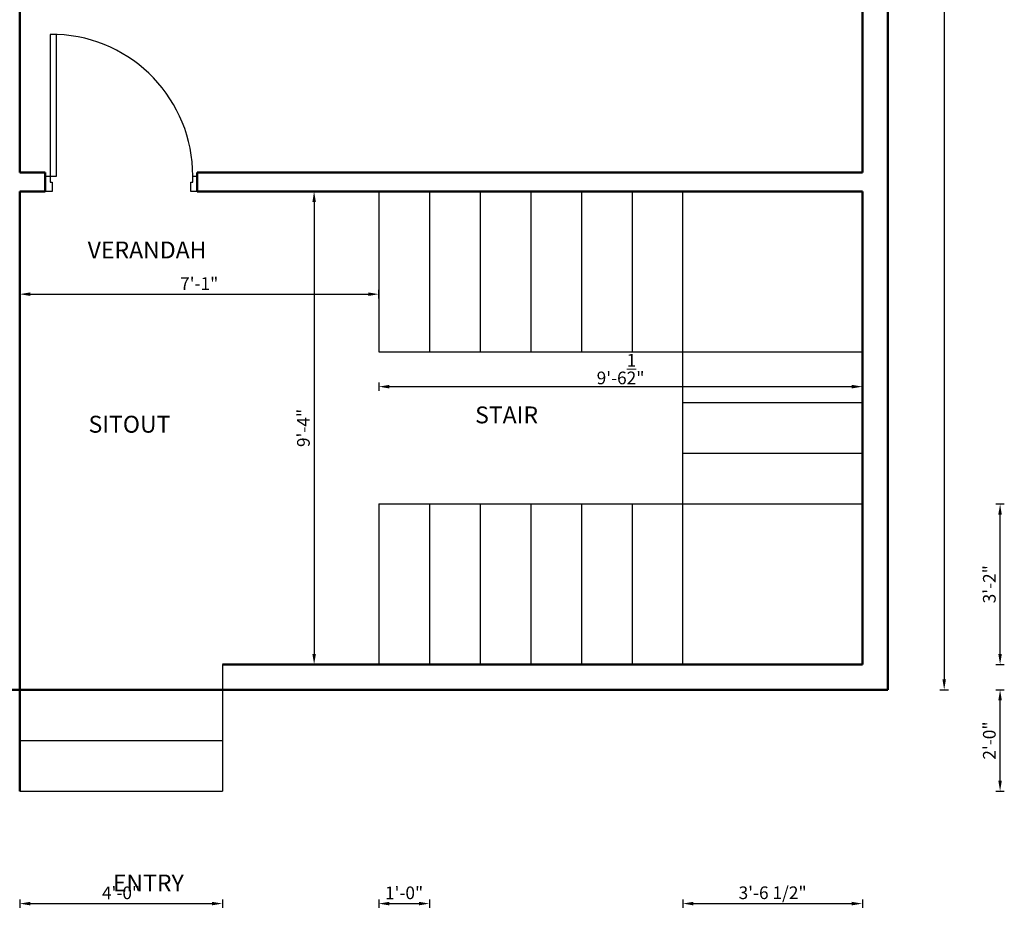
# Model space of a CAD drawing. Units: inches. Extents: x 1961 to 3038, y 800 to 1438.
# Tile 6 of 13: x 2803 to 3036, y 800 to 1012. Entities that reach past the tile are written whole.
import ezdxf

# ---------------------------------------------------------------- set-up
doc = ezdxf.new("R2010")
doc.units = ezdxf.units.IN
for name, color, linetype, lineweight in [('A-ANNO-DIMS', 2, 'Continuous', 18), ('A-ANNO-TEXT', 7, 'Continuous', 25), ('A-AREA-IDEN', 7, 'Continuous', 25), ('A-DOOR', 3, 'Continuous', 25), ('A-FLOR-STRS', 7, 'Continuous', 25), ('A-WALL', 7, 'Continuous', 50)]:
    doc.layers.add(name, color=color, linetype=linetype, lineweight=lineweight)
doc.styles.get("Standard").update_dxf_attribs({"font": 'arial.ttf'})
doc.dimstyles.new('ISO-25', dxfattribs={"dimtxt": 3, "dimasz": 2.5, "dimexe": 1, "dimexo": 1, "dimtad": 1, "dimdec": 4, "dimlunit": 4, "dimtxsty": 'Standard', "dimcen": 2.5, "dimadec": 0, "dimazin": 0, "dimtfac": 1, "dimtdec": 4, "dimtmove": 0, "dimatfit": 3, "dimfxl": 1, "dimfxlon": 1, "dimarcsym": 0})

# ---------------------------------------------------------------- blocks, each defined once
blk = doc.blocks.new('*D6')
at = {"layer": 'A-ANNO-DIMS', "color": 0, "lineweight": -2, "transparency": 16777216}
for p, q in [((2873.97, 970.92), (2871.97, 970.92)), ((2872.97, 968.42), (2872.97, 861.42)), ((2873.97, 858.92), (2871.97, 858.92))]:
    blk.add_line(p, q, dxfattribs=at)
at = {"layer": 'A-ANNO-DIMS', "color": 0, "transparency": 16777216}
for points in [[(2872.56, 968.42), (2873.39, 968.42), (2872.97, 970.92)], [(2872.56, 861.42), (2873.39, 861.42), (2872.97, 858.92)]]:
    blk.add_solid(points, dxfattribs=at)
at = {"layer": 'Defpoints', "color": 0, "transparency": 16777216}
for p in [(2888.27, 970.92), (2872.97, 858.92), (2888.27, 858.92)]:
    blk.add_point(p, dxfattribs=at)
at = {"layer": 'A-ANNO-DIMS', "color": 0, "transparency": 16777216, "insert": (2870.82, 914.92), "char_height": 3, "attachment_point": 5, "rotation": 90}
blk.add_mtext('9\'-4"', dxfattribs=at)
blk = doc.blocks.new('*D7')
at = {"layer": 'A-ANNO-DIMS', "color": 0, "lineweight": -2, "transparency": 16777216}
for p, q in [((2803.27, 945.9), (2803.27, 947.59)), ((2805.77, 946.59), (2885.77, 946.59)), ((2888.27, 945.59), (2888.27, 947.59))]:
    blk.add_line(p, q, dxfattribs=at)
at = {"layer": 'A-ANNO-DIMS', "color": 0, "transparency": 16777216}
for points in [[(2805.77, 947.01), (2805.77, 946.17), (2803.27, 946.59)], [(2885.77, 947.01), (2885.77, 946.17), (2888.27, 946.59)]]:
    blk.add_solid(points, dxfattribs=at)
at = {"layer": 'Defpoints', "color": 0, "transparency": 16777216}
for p in [(2888.27, 946.59), (2803.27, 944.9), (2888.27, 943.36)]:
    blk.add_point(p, dxfattribs=at)
at = {"layer": 'A-ANNO-DIMS', "color": 0, "transparency": 16777216, "insert": (2845.77, 948.72), "char_height": 3, "attachment_point": 5}
blk.add_mtext('7\'-1"', dxfattribs=at)
blk = doc.blocks.new('*D8')
at = {"layer": 'A-ANNO-DIMS', "color": 0, "lineweight": -2, "transparency": 16777216}
for p, q in [((2888.27, 925.7), (2888.27, 923.7)), ((3002.77, 925.7), (3002.77, 923.7)), ((2890.77, 924.7), (3000.27, 924.7))]:
    blk.add_line(p, q, dxfattribs=at)
at = {"layer": 'A-ANNO-DIMS', "color": 0, "transparency": 16777216}
for points in [[(2890.77, 925.12), (2890.77, 924.28), (2888.27, 924.7)], [(3000.27, 925.12), (3000.27, 924.28), (3002.77, 924.7)]]:
    blk.add_solid(points, dxfattribs=at)
at = {"layer": 'Defpoints', "color": 0, "transparency": 16777216}
for p in [(2888.27, 932.92), (3002.77, 932.92), (3002.77, 924.7)]:
    blk.add_point(p, dxfattribs=at)
at = {"layer": 'A-ANNO-DIMS', "color": 0, "transparency": 16777216, "insert": (2945.52, 928.86), "char_height": 3, "attachment_point": 5}
blk.add_mtext('9\'-6{\\H1x;\\S1/2;}"', dxfattribs=at)
blk = doc.blocks.new('*D26')
at = {"layer": 'A-ANNO-DIMS', "color": 0, "lineweight": -2, "transparency": 16777216}
for p, q in [((3021.14, 1314.92), (3023.14, 1314.92)), ((3022.14, 1312.42), (3022.14, 855.42)), ((3021.14, 852.92), (3023.14, 852.92))]:
    blk.add_line(p, q, dxfattribs=at)
at = {"layer": 'A-ANNO-DIMS', "color": 0, "transparency": 16777216}
for points in [[(3021.72, 1312.42), (3022.55, 1312.42), (3022.14, 1314.92)], [(3021.72, 855.42), (3022.55, 855.42), (3022.14, 852.92)]]:
    blk.add_solid(points, dxfattribs=at)
at = {"layer": 'Defpoints', "color": 0, "transparency": 16777216}
for p in [(3008.77, 1314.92), (3008.77, 852.92), (3022.14, 852.92)]:
    blk.add_point(p, dxfattribs=at)
at = {"layer": 'A-ANNO-DIMS', "color": 0, "transparency": 16777216, "insert": (3019.98, 1083.92), "char_height": 3, "attachment_point": 5, "rotation": 90}
blk.add_mtext('38\'-6"', dxfattribs=at)
blk = doc.blocks.new('*D71')
at = {"layer": 'A-ANNO-DIMS', "color": 0, "lineweight": -2, "transparency": 16777216}
for p, q in [((2803.27, 803.32), (2803.27, 801.32)), ((2805.77, 802.32), (2848.77, 802.32)), ((2851.27, 803.32), (2851.27, 801.32))]:
    blk.add_line(p, q, dxfattribs=at)
at = {"layer": 'A-ANNO-DIMS', "color": 0, "transparency": 16777216}
for points in [[(2805.77, 802.74), (2805.77, 801.9), (2803.27, 802.32)], [(2848.77, 802.74), (2848.77, 801.9), (2851.27, 802.32)]]:
    blk.add_solid(points, dxfattribs=at)
at = {"layer": 'Defpoints', "color": 0, "transparency": 16777216}
for p in [(2803.27, 828.92), (2851.27, 828.92), (2851.27, 802.32)]:
    blk.add_point(p, dxfattribs=at)
at = {"layer": 'A-ANNO-DIMS', "color": 0, "transparency": 16777216, "insert": (2827.27, 804.48), "char_height": 3, "attachment_point": 5}
blk.add_mtext('4\'-0"', dxfattribs=at)
blk = doc.blocks.new('*D72')
at = {"layer": 'A-ANNO-DIMS', "color": 0, "lineweight": -2, "transparency": 16777216}
for p, q in [((3034.37, 852.92), (3036.37, 852.92)), ((3035.37, 831.42), (3035.37, 850.42)), ((3034.37, 828.92), (3036.37, 828.92))]:
    blk.add_line(p, q, dxfattribs=at)
at = {"layer": 'A-ANNO-DIMS', "color": 0, "transparency": 16777216}
for points in [[(3034.95, 850.42), (3035.78, 850.42), (3035.37, 852.92)], [(3034.95, 831.42), (3035.78, 831.42), (3035.37, 828.92)]]:
    blk.add_solid(points, dxfattribs=at)
at = {"layer": 'Defpoints', "color": 0, "transparency": 16777216}
for p in [(3008.77, 852.92), (3035.37, 852.92), (2851.27, 828.92)]:
    blk.add_point(p, dxfattribs=at)
at = {"layer": 'A-ANNO-DIMS', "color": 0, "transparency": 16777216, "insert": (3033.21, 840.92), "char_height": 3, "attachment_point": 5, "rotation": 90}
blk.add_mtext('2\'-0"', dxfattribs=at)
blk = doc.blocks.new('*D75')
at = {"layer": 'A-ANNO-DIMS', "color": 0, "lineweight": -2, "transparency": 16777216}
for p, q in [((2809.27, 1340.52), (2809.27, 1342.52)), ((2811.77, 1341.52), (2842.77, 1341.52)), ((2845.27, 1340.52), (2845.27, 1342.52))]:
    blk.add_line(p, q, dxfattribs=at)
at = {"layer": 'A-ANNO-DIMS', "color": 0, "transparency": 16777216}
for points in [[(2811.77, 1341.94), (2811.77, 1341.1), (2809.27, 1341.52)], [(2842.77, 1341.94), (2842.77, 1341.1), (2845.27, 1341.52)]]:
    blk.add_solid(points, dxfattribs=at)
at = {"layer": 'Defpoints', "color": 0, "transparency": 16777216}
for p in [(2845.27, 1341.52), (2809.27, 970.92), (2845.27, 970.92)]:
    blk.add_point(p, dxfattribs=at)
at = {"layer": 'A-ANNO-DIMS', "color": 0, "transparency": 16777216, "insert": (2827.27, 1343.68), "char_height": 3, "attachment_point": 5}
blk.add_mtext('3\'-0"', dxfattribs=at)
blk = doc.blocks.new('*D88')
at = {"layer": 'A-ANNO-DIMS', "color": 0, "lineweight": -2, "transparency": 16777216}
for p, q in [((2888.27, 803.32), (2888.27, 801.32)), ((2890.77, 802.32), (2897.77, 802.32)), ((2900.27, 803.32), (2900.27, 801.32))]:
    blk.add_line(p, q, dxfattribs=at)
at = {"layer": 'A-ANNO-DIMS', "color": 0, "transparency": 16777216}
for points in [[(2890.77, 802.74), (2890.77, 801.9), (2888.27, 802.32)], [(2897.77, 802.74), (2897.77, 801.9), (2900.27, 802.32)]]:
    blk.add_solid(points, dxfattribs=at)
at = {"layer": 'Defpoints', "color": 0, "transparency": 16777216}
for p in [(2888.27, 858.92), (2900.27, 858.92), (2900.27, 802.32)]:
    blk.add_point(p, dxfattribs=at)
at = {"layer": 'A-ANNO-DIMS', "color": 0, "transparency": 16777216, "insert": (2894.27, 804.48), "char_height": 3, "attachment_point": 5}
blk.add_mtext('1\'-0"', dxfattribs=at)
blk = doc.blocks.new('*D89')
at = {"layer": 'A-ANNO-DIMS', "color": 0, "lineweight": -2, "transparency": 16777216}
for p, q in [((3034.37, 896.92), (3036.37, 896.92)), ((3035.37, 861.42), (3035.37, 894.42)), ((3034.37, 858.92), (3036.37, 858.92))]:
    blk.add_line(p, q, dxfattribs=at)
at = {"layer": 'A-ANNO-DIMS', "color": 0, "transparency": 16777216}
for points in [[(3034.95, 894.42), (3035.78, 894.42), (3035.37, 896.92)], [(3034.95, 861.42), (3035.78, 861.42), (3035.37, 858.92)]]:
    blk.add_solid(points, dxfattribs=at)
at = {"layer": 'Defpoints', "color": 0, "transparency": 16777216}
for p in [(3002.77, 896.92), (3035.37, 896.92), (3002.77, 858.92)]:
    blk.add_point(p, dxfattribs=at)
at = {"layer": 'A-ANNO-DIMS', "color": 0, "transparency": 16777216, "insert": (3033.21, 877.92), "char_height": 3, "attachment_point": 5, "rotation": 90}
blk.add_mtext('3\'-2"', dxfattribs=at)
blk = doc.blocks.new('*D90')
at = {"layer": 'A-ANNO-DIMS', "color": 0, "lineweight": -2, "transparency": 16777216}
for p, q in [((2960.27, 803.32), (2960.27, 801.32)), ((2962.77, 802.32), (3000.27, 802.32)), ((3002.77, 803.32), (3002.77, 801.32))]:
    blk.add_line(p, q, dxfattribs=at)
at = {"layer": 'A-ANNO-DIMS', "color": 0, "transparency": 16777216}
for points in [[(2962.77, 802.74), (2962.77, 801.9), (2960.27, 802.32)], [(3000.27, 802.74), (3000.27, 801.9), (3002.77, 802.32)]]:
    blk.add_solid(points, dxfattribs=at)
at = {"layer": 'Defpoints', "color": 0, "transparency": 16777216}
for p in [(2960.27, 858.92), (3002.77, 858.92), (3002.77, 802.32)]:
    blk.add_point(p, dxfattribs=at)
at = {"layer": 'A-ANNO-DIMS', "color": 0, "transparency": 16777216, "insert": (2981.52, 804.5), "char_height": 3, "attachment_point": 5}
blk.add_mtext('3\'-6 1/2"', dxfattribs=at)

msp = doc.modelspace()

# ---------------------------------------------------------------- linework, layer by layer
at = {"layer": 'A-DOOR'}
for p, q in [((2812.15182, 1008.09185), (2810.50415, 1008.09185)), ((2810.50415, 1008.09185), (2810.50415, 974.56408)), ((2811.96188, 974.56408), (2811.96188, 1008.09185)), ((2809.26803, 974.56408), (2811.96188, 974.56408)), ((2810.50415, 974.56408), (2810.50415, 973.10635)), ((2810.50415, 973.10635), (2810.94738, 973.10635)), ((2810.94738, 973.10635), (2810.94738, 970.91975)), ((2810.94738, 970.91975), (2809.26803, 970.91975))]:
    msp.add_line(p, q, dxfattribs=at)
msp.add_lwpolyline([(2845.26803, 970.91975), (2843.8103, 970.91975), (2843.8103, 973.10635), (2844.25353, 973.10635), (2844.25353, 974.56408), (2845.26803, 974.56408)], dxfattribs=at)
msp.add_arc((2810.69409, 974.56408), 33.55944, 0, 87.5104471, dxfattribs=at)
at = {"layer": 'A-FLOR-STRS'}
for p, q in [((2888.26803, 970.91975), (2888.26803, 932.91975)), ((2900.26803, 970.91975), (2900.26803, 932.91975)), ((2912.26803, 970.91975), (2912.26803, 932.91975)), ((2924.26803, 970.91975), (2924.26803, 932.91975)), ((2936.26803, 970.91975), (2936.26803, 932.91975)), ((2948.26803, 970.91975), (2948.26803, 932.91975)), ((2960.26803, 858.91975), (2960.26803, 970.91975)), ((2888.26803, 932.91975), (3002.76803, 932.91975)), ((2960.26803, 920.91975), (3002.76803, 920.91975)), ((2960.26803, 908.91975), (3002.76803, 908.91975)), ((2888.26803, 896.91975), (3002.76803, 896.91975)), ((2888.26803, 896.91975), (2888.26803, 858.91975)), ((2900.26803, 896.91975), (2900.26803, 858.91975)), ((2912.26803, 896.91975), (2912.26803, 858.91975)), ((2924.26803, 896.91975), (2924.26803, 858.91975)), ((2936.26803, 896.91975), (2936.26803, 858.91975)), ((2948.26803, 896.91975), (2948.26803, 858.91975)), ((2851.26803, 858.91975), (2851.26803, 828.91975)), ((2803.26803, 840.91975), (2851.26803, 840.91975)), ((2803.26803, 828.91975), (2851.26803, 828.91975))]:
    msp.add_line(p, q, dxfattribs=at)
at = {"layer": 'A-WALL'}
for p, q in [((3008.76803, 852.91975), (3008.76803, 1314.91975)), ((3002.76803, 975.41975), (3002.76803, 1160.41975)), ((2803.26803, 1058.41975), (2803.26803, 975.41975)), ((2803.26803, 975.41975), (2809.26803, 975.41975)), ((2809.26803, 975.41975), (2809.26803, 970.91975)), ((2845.26803, 975.41975), (2845.26803, 970.91975)), ((2845.26803, 975.41975), (3002.76803, 975.41975)), ((2803.26803, 970.91975), (2809.26803, 970.91975)), ((2803.26803, 970.91975), (2803.26803, 828.91975)), ((2845.26803, 970.91975), (3002.76803, 970.91975)), ((3002.76803, 858.91975), (3002.76803, 970.91975)), ((2851.26803, 858.91975), (3002.76803, 858.91975)), ((2624.76803, 852.91975), (3008.76803, 852.91975))]:
    msp.add_line(p, q, dxfattribs=at)

# ---------------------------------------------------------------- texts
at = {"layer": 'A-ANNO-TEXT', "insert": (2825.32477, 809.19736), "char_height": 4, "attachment_point": 1}
msp.add_mtext_dynamic_manual_height_columns('{\\fTimes New Roman|b1|i0|c0|p18;ENTRY}', width=33.1080891, gutter_width=12.5, heights=[0], dxfattribs=at)
at = {"layer": 'A-AREA-IDEN', "char_height": 4, "attachment_point": 1}
for s, insert in [('{\\fTimes New Roman|b1|i0|c0|p18;VERANDAH}', (2819.35929, 959.05988)), ('{\\fTimes New Roman|b1|i0|c0|p18;STAIR}', (2911.08473, 920.00906)), ('{\\fTimes New Roman|b1|i0|c0|p18;SITOUT}', (2819.5714, 917.80227))]:
    msp.add_mtext_dynamic_manual_height_columns(s, width=33.1080891, gutter_width=12.5, heights=[0], dxfattribs=dict(at, insert=insert))

# ---------------------------------------------------------------- dimensions: what is measured, and where the dimension line sits
at = {"layer": 'A-ANNO-DIMS'}
for base, p1, p2, override, picture, middle in [((2845.26803, 1341.51975), (2809.26803, 970.91975), (2845.26803, 970.91975), {"dimdec": 1, "dimlfac": 1, "dimrnd": 0, "dimzin": 1, "dimdsep": 46, "dimlunit": 4, "dimfrac": 2}, '*D75', (2827.26803, 1343.6775)), ((2888.26803, 946.59022), (2803.26803, 944.90467), (2888.26803, 943.35958), {"dimclrd": 0, "dimclre": 0, "dimclrt": 0}, '*D7', (2845.76803, 948.72136)), ((3002.76803, 924.69984), (2888.26803, 932.91975), (3002.76803, 932.91975), {"dimclrd": 0, "dimclre": 0, "dimclrt": 0}, '*D8', (2945.51803, 928.8627)), ((2900.26803, 802.31975), (2888.26803, 858.91975), (2900.26803, 858.91975), {"dimdec": 1, "dimlfac": 1, "dimrnd": 0, "dimzin": 1, "dimdsep": 46, "dimlunit": 4, "dimfrac": 2}, '*D88', (2894.26803, 804.47647)), ((3002.76803, 802.31975), (2960.26803, 858.91975), (3002.76803, 858.91975), {"dimdec": 1, "dimlfac": 1, "dimrnd": 0, "dimzin": 1, "dimdsep": 46, "dimlunit": 4, "dimfrac": 2}, '*D90', (2981.51803, 804.49694)), ((2851.26803, 802.31975), (2803.26803, 828.91975), (2851.26803, 828.91975), {"dimdec": 1, "dimlfac": 1, "dimrnd": 0, "dimzin": 1, "dimdsep": 46, "dimlunit": 4, "dimfrac": 2}, '*D71', (2827.26803, 804.47647))]:
    dim = msp.add_linear_dim(base=base, p1=p1, p2=p2, dimstyle='ISO-25', override=override, dxfattribs=at)
    dim.commit()
    dim.dimension.update_dxf_attribs({"geometry": picture, "text_midpoint": middle})
for base, p1, p2, override, picture, middle in [((3022.1353, 852.91975), (3008.76803, 1314.91975), (3008.76803, 852.91975), {"dimclrd": 0, "dimclre": 0, "dimclrt": 0}, '*D26', (3019.97756, 1083.91975)), ((2872.9718, 858.91975), (2888.26803, 970.91975), (2888.26803, 858.91975), {"dimclrd": 0, "dimclre": 0, "dimclrt": 0}, '*D6', (2870.81508, 914.91975)), ((3035.36803, 896.91975), (3002.76803, 858.91975), (3002.76803, 896.91975), {"dimdec": 1, "dimlfac": 1, "dimrnd": 0, "dimzin": 1, "dimdsep": 46, "dimlunit": 4, "dimfrac": 2}, '*D89', (3033.21029, 877.91975)), ((3035.36803, 852.91975), (2851.26803, 828.91975), (3008.76803, 852.91975), {"dimdec": 1, "dimlfac": 1, "dimrnd": 0, "dimzin": 1, "dimdsep": 46, "dimlunit": 4, "dimfrac": 2}, '*D72', (3033.21131, 840.91975))]:
    dim = msp.add_linear_dim(base=base, p1=p1, p2=p2, angle=90, dimstyle='ISO-25', override=override, dxfattribs=at)
    dim.commit()
    dim.dimension.update_dxf_attribs({"geometry": picture, "text_midpoint": middle})

doc.saveas('drawing.dxf')
